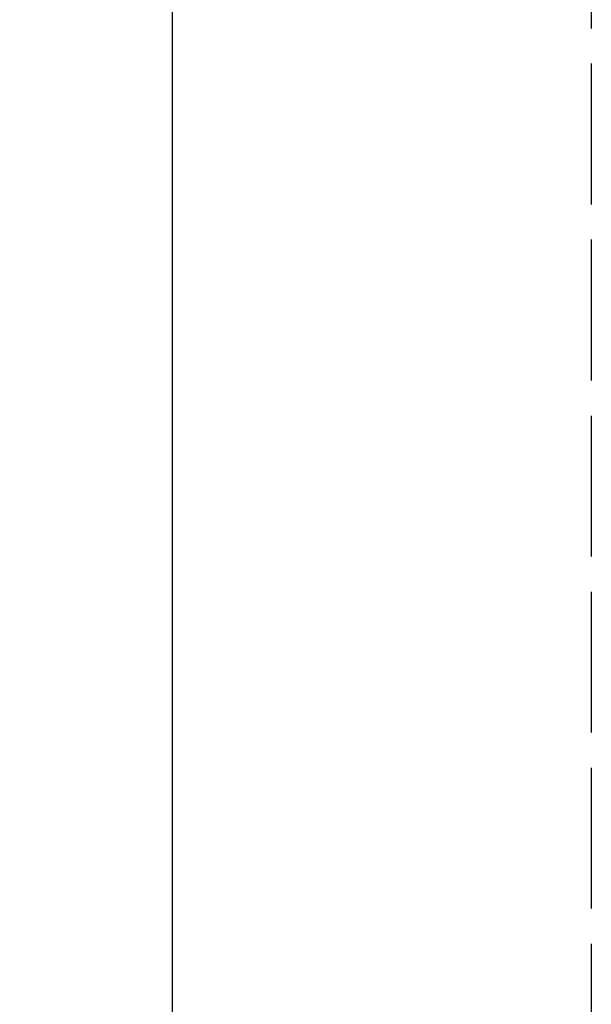
# Model space of a CAD drawing. Units: inches. Extents: x 1316 to 1777, y 813 to 1650.
# Tile 6 of 22: x 1316 to 1364, y 1284 to 1368. Entities that reach past the tile are written whole.
import ezdxf

# ---------------------------------------------------------------- set-up
doc = ezdxf.new("R2010")
doc.units = ezdxf.units.IN
doc.header["$MEASUREMENT"] = 0
doc.linetypes.add('ACAD_ISO02W100', pattern=[15, 12, -3])
doc.layers.add('A-ANNO-DIMS', color=2, linetype='Continuous', lineweight=18)
doc.layers.add('C-PROP', color=8, linetype='ACAD_ISO02W100', lineweight=25)
doc.styles.get("Standard").update_dxf_attribs({"font": 'arial.ttf'})
doc.dimstyles.get("Standard").update_dxf_attribs({"dimtxt": 7, "dimasz": 0.18, "dimexe": 0.18, "dimexo": 0.0625, "dimgap": 0.09, "dimtad": 0, "dimtih": 1, "dimtoh": 1, "dimzin": 0, "dimdsep": 46, "dimlunit": 3, "dimtxsty": 'Standard', "dimcen": 0.09, "dimadec": 0, "dimazin": 0, "dimtfac": 1, "dimtofl": 0, "dimtmove": 0, "dimatfit": 3, "dimfxl": 1, "dimtolj": 1, "dimtzin": 0, "dimarcsym": 0})

# ---------------------------------------------------------------- blocks, each defined once
blk = doc.blocks.new('*D23')
at = {"layer": 'A-ANNO-DIMS', "color": 0, "lineweight": -2, "transparency": 16777216}
for p, q in [((1328.466746604303, 1604.172951843256), (1328.865516882555, 1604.172951843256)), ((1328.685516882555, 1603.992951843256), (1328.685516882555, 1282.594977494184)), ((1328.685516882555, 953.868981317008), (1328.685516882555, 1275.26695566608)), ((1328.466746604303, 953.688981317008), (1328.865516882556, 953.688981317008))]:
    blk.add_line(p, q, dxfattribs=at)
at = {"layer": 'A-ANNO-DIMS', "color": 0, "transparency": 16777216}
for points in [[(1328.655516882555, 1603.992951843256), (1328.715516882555, 1603.992951843256), (1328.685516882555, 1604.172951843256)], [(1328.655516882556, 953.868981317008), (1328.715516882555, 953.868981317008), (1328.685516882555, 953.688981317008)]]:
    blk.add_solid(points, dxfattribs=at)
at = {"layer": 'Defpoints', "color": 0, "transparency": 16777216}
for p in [(1328.404246604303, 1604.172951843256), (1328.404246604303, 953.688981317008), (1328.685516882555, 953.688981317008)]:
    blk.add_point(p, dxfattribs=at)
at = {"layer": 'A-ANNO-DIMS', "color": 0, "transparency": 16777216, "insert": (1328.685516882555, 1278.930966580132), "char_height": 7, "width": 24.3281036834925, "attachment_point": 5}
blk.add_mtext('\\A1;47\'-0"', dxfattribs=at)

msp = doc.modelspace()

# ---------------------------------------------------------------- linework, layer by layer
at = {"layer": 'C-PROP'}
msp.add_line((1364.398563382318, 1604.172951843256), (1364.398563382318, 953.6889813170072), dxfattribs=at)

# ---------------------------------------------------------------- dimensions: what is measured, and where the dimension line sits
at = {"layer": 'A-ANNO-DIMS'}
dim = msp.add_linear_dim(base=(1328.685516882555, 953.688981317008), p1=(1328.404246604303, 1604.172951843256), p2=(1328.404246604303, 953.6889813170077), angle=90, text='47\'-0"', dimstyle='Standard', override={"dimclrd": 0, "dimclre": 0, "dimclrt": 0}, dxfattribs=at)
dim.commit()
dim.dimension.update_dxf_attribs({"geometry": '*D23', "text_midpoint": (1328.685516882555, 1278.930966580132)})

doc.saveas('drawing.dxf')
